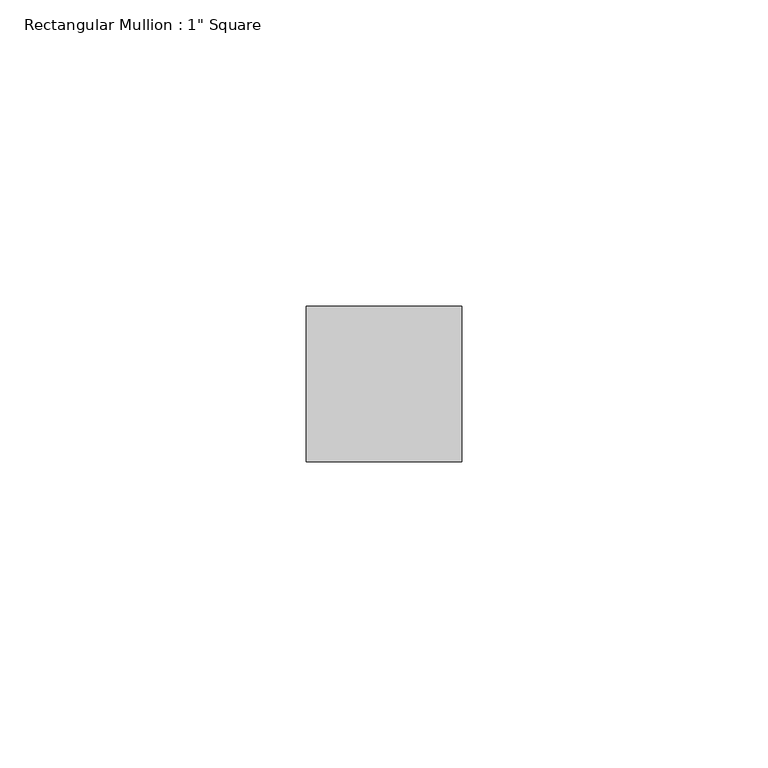
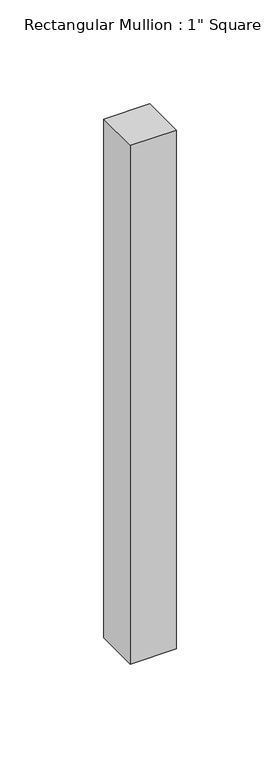
"""IFC4 building model written with IfcOpenShell, lengths in millimetres: member geometry."""

from ifc_helpers import new_model, si_unit, frame, origin, place, context, project, spatial, polyline, outline, extrude, source, transform, mapped, element, save


def member_839e3c67(model_context):
    return source(origin(), model_context, "Body", "SweptSolid", [
        extrude(outline(polyline([(0.0, 12.7), (0.0, -12.7), (-25.4, -12.7), (-25.4, 12.7), (0.0, 12.7)])), frame((0.0, 0.0, -304.8), z_axis=(0.0, 0.0, 1.0), x_axis=(1.0, 0.0, 0.0)), (0.0, 0.0, 1.0), 304.8),
    ])


if __name__ == "__main__":
    model = new_model("IFC4")
    model_context = context("Model", 3, world=origin())
    ifc_project = project(units=[si_unit("LENGTHUNIT", "METRE", prefix="MILLI")], contexts=[model_context])
    site = spatial("IfcSite", under=ifc_project)
    building = spatial("IfcBuilding", under=site)
    placement = place(None, origin())
    member_shape = member_839e3c67(model_context)
    element("IfcMember", 1, ObjectType="Rectangular Mullion : 1\" Square", at=placement, inside=building, context=model_context, shape_type="MappedRepresentation", body=[
        mapped(member_shape, transform((0.0, 0.0, 0.0), x_axis=(1.0, 0.0, 0.0), y_axis=(0.0, 1.0, 0.0), z_axis=(0.0, 0.0, 1.0))),
    ])
    save(model, "model.ifc")

# Revit data of these elements
# Type "Rectangular Mullion : 1\" Square"
#   built-in parameter 1007304 = 0.0833333 (stored number, unit not read)
#   built-in parameter 1007301 = 0.0416667 (stored number, unit not read)
#   built-in parameter 1007300 = 0.0416667 (stored number, unit not read)
